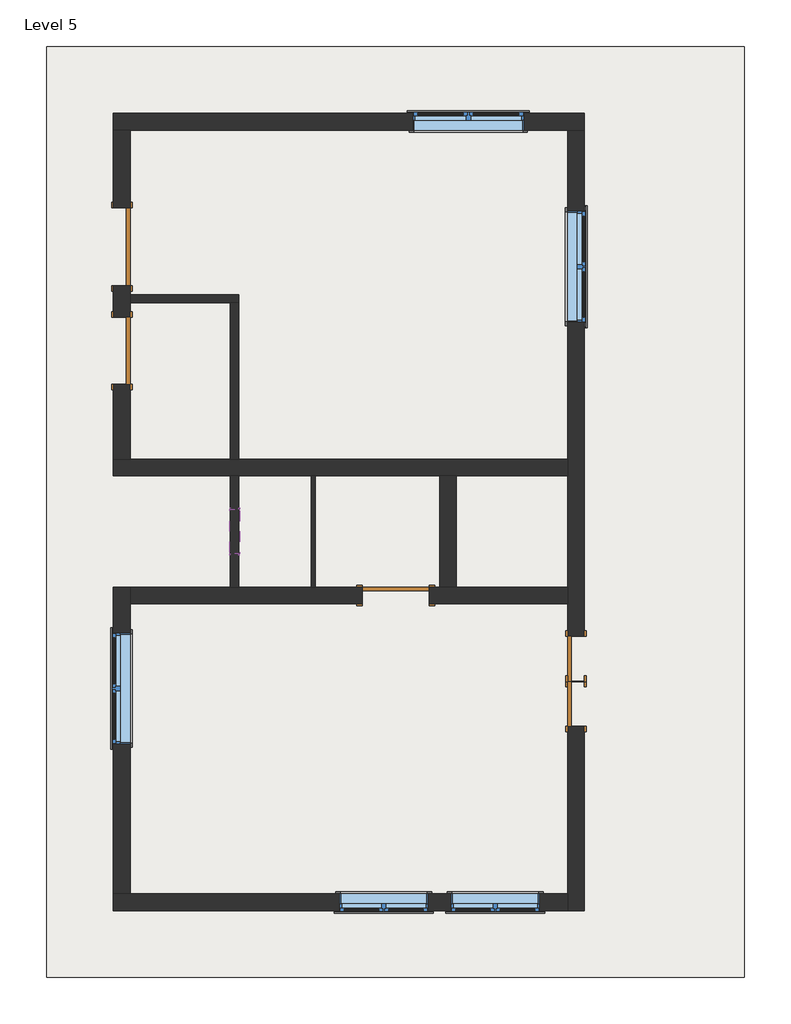
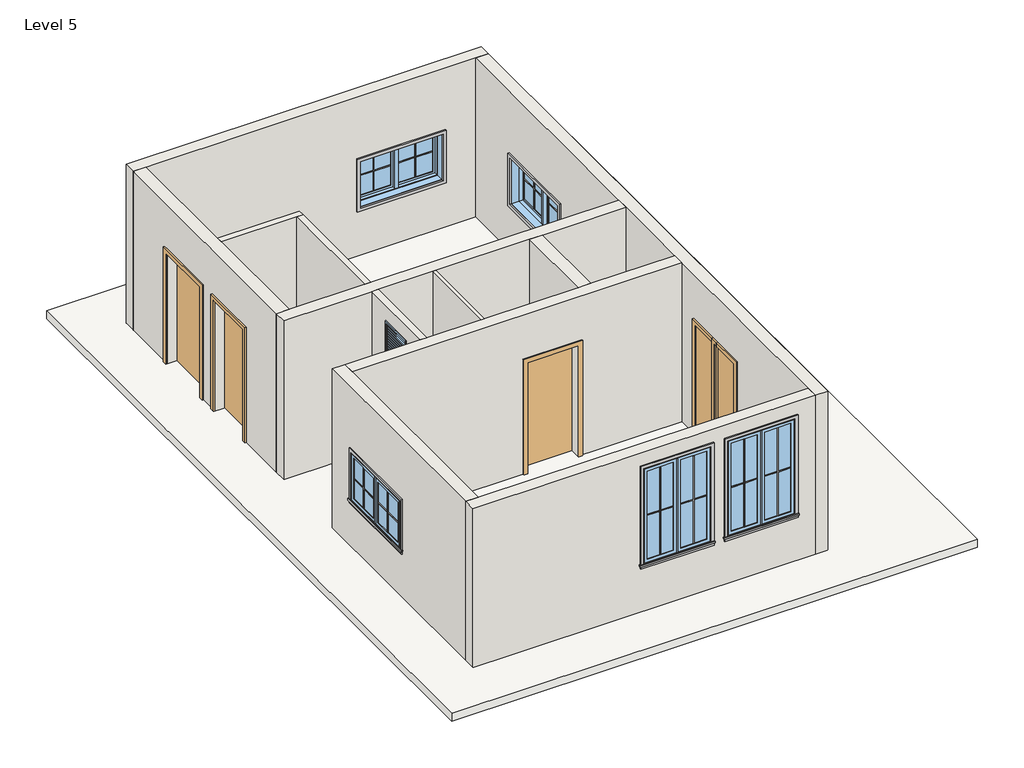
# One storey, incomplete: 20 proxies, 12 walls, 6 windows, 5 doors, 1 roof.
"""IFC4 building model written with IfcOpenShell, lengths in millimetres."""

from ifc_helpers import new_model, si_unit, frame, origin, place, context, project, spatial, polyline, outline, extrude, faceted_brep, transform, mapped, element, save
from components import muntin_pattern_2x2_muntin_pattern_2x2_9352d081, muntin_pattern_2x2_muntin_pattern_2x2_5c2cbe28, muntin_pattern_2x2_muntin_pattern_2x2_2b4d9f72, muntin_pattern_2x2_muntin_pattern_2x2_ef995ed3, trim_window_exterior_flat_with_sill_979bde60, trim_window_exterior_flat_with_sill_b7e4d11c, trim_window_interior_flat_picture_frame_7883d11b, trim_window_interior_flat_picture_frame_936b8d2a, single_flush_door_2_0d3b4037, single_flush_door_2_4a3212df, door_a90ba1ad, door_0ca8825f, door_9d399b00, window_casement_double_c1d95f0f, window_casement_double_wall_4_6ca1769e, window_d39e7ecb

model = new_model("IFC4")

# Units and contexts
model_context = context("Model", 3, world=origin())
ifc_project = project(units=[si_unit("LENGTHUNIT", "METRE", prefix="MILLI")], contexts=[model_context])

# Site, building, storey
site = spatial("IfcSite", under=ifc_project)
building = spatial("IfcBuilding", under=site)
storey = spatial("IfcBuildingStorey", under=building, Name="Level 5", Elevation=9601.2)

# Proxies
placement = place(None, origin())
muntin_pattern_2x2_muntin_pattern_2x2_shape = muntin_pattern_2x2_muntin_pattern_2x2_9352d081(model_context)
element("IfcBuildingElementProxy", 1, Name="Muntin Pattern_2x2 : Muntin Pattern_2x2", ObjectType="Muntin Pattern_2x2 : Muntin Pattern_2x2", at=placement, inside=storey, context=model_context, shape_type="MappedRepresentation", body=[
    mapped(muntin_pattern_2x2_muntin_pattern_2x2_shape, transform((-4785.3510342, -2707.8617544, 10585.45), x_axis=(0.0, 1.0, 0.0), y_axis=(-1.0, 0.0, 0.0), z_axis=(0.0, 0.0, 1.0))),
])
element("IfcBuildingElementProxy", 2, Name="Muntin Pattern_2x2 : Muntin Pattern_2x2", ObjectType="Muntin Pattern_2x2 : Muntin Pattern_2x2", at=placement, inside=storey, context=model_context, shape_type="MappedRepresentation", body=[
    mapped(muntin_pattern_2x2_muntin_pattern_2x2_shape, transform((1634.4989658, 3816.7632456, 10585.45), x_axis=(0.0, -1.0, 0.0), y_axis=(1.0, 0.0, 0.0), z_axis=(0.0, 0.0, 1.0))),
])
element("IfcBuildingElementProxy", 3, Name="Muntin Pattern_2x2 : Muntin Pattern_2x2", ObjectType="Muntin Pattern_2x2 : Muntin Pattern_2x2", at=placement, inside=storey, context=model_context, shape_type="MappedRepresentation", body=[
    mapped(muntin_pattern_2x2_muntin_pattern_2x2_shape, transform((-322.8885342, 5523.3257456, 10585.45), x_axis=(1.0, 0.0, 0.0), y_axis=(0.0, 1.0, 0.0), z_axis=(0.0, 0.0, 1.0))),
])
muntin_pattern_2x2_muntin_pattern_2x2_2_shape = muntin_pattern_2x2_muntin_pattern_2x2_5c2cbe28(model_context)
element("IfcBuildingElementProxy", 4, Name="Muntin Pattern_2x2 : Muntin Pattern_2x2", ObjectType="Muntin Pattern_2x2 : Muntin Pattern_2x2", at=placement, inside=storey, context=model_context, shape_type="MappedRepresentation", body=[
    mapped(muntin_pattern_2x2_muntin_pattern_2x2_2_shape, transform((-4785.3510342, -1949.0367544, 10585.45), x_axis=(0.0, -1.0, 0.0), y_axis=(1.0, 0.0, 0.0), z_axis=(0.0, 0.0, 1.0))),
])
element("IfcBuildingElementProxy", 5, Name="Muntin Pattern_2x2 : Muntin Pattern_2x2", ObjectType="Muntin Pattern_2x2 : Muntin Pattern_2x2", at=placement, inside=storey, context=model_context, shape_type="MappedRepresentation", body=[
    mapped(muntin_pattern_2x2_muntin_pattern_2x2_2_shape, transform((1634.4989658, 3057.9382456, 10585.45), x_axis=(0.0, 1.0, 0.0), y_axis=(-1.0, 0.0, 0.0), z_axis=(0.0, 0.0, 1.0))),
])
element("IfcBuildingElementProxy", 6, Name="Muntin Pattern_2x2 : Muntin Pattern_2x2", ObjectType="Muntin Pattern_2x2 : Muntin Pattern_2x2", at=placement, inside=storey, context=model_context, shape_type="MappedRepresentation", body=[
    mapped(muntin_pattern_2x2_muntin_pattern_2x2_2_shape, transform((435.9364658, 5523.3257456, 10585.45), x_axis=(-1.0, 0.0, 0.0), y_axis=(0.0, -1.0, 0.0), z_axis=(0.0, 0.0, 1.0))),
])
muntin_pattern_2x2_muntin_pattern_2x2_3_shape = muntin_pattern_2x2_muntin_pattern_2x2_2b4d9f72(model_context)
element("IfcBuildingElementProxy", 7, Name="Muntin Pattern_2x2 : Muntin Pattern_2x2", ObjectType="Muntin Pattern_2x2 : Muntin Pattern_2x2", at=placement, inside=storey, context=model_context, shape_type="MappedRepresentation", body=[
    mapped(muntin_pattern_2x2_muntin_pattern_2x2_3_shape, transform((-795.9635342, -5354.2242544, 10585.45), x_axis=(-1.0, 0.0, 0.0), y_axis=(0.0, -1.0, 0.0), z_axis=(0.0, 0.0, 1.0))),
])
element("IfcBuildingElementProxy", 8, Name="Muntin Pattern_2x2 : Muntin Pattern_2x2", ObjectType="Muntin Pattern_2x2 : Muntin Pattern_2x2", at=placement, inside=storey, context=model_context, shape_type="MappedRepresentation", body=[
    mapped(muntin_pattern_2x2_muntin_pattern_2x2_3_shape, transform((728.0364658, -5354.2242544, 10585.45), x_axis=(-1.0, 0.0, 0.0), y_axis=(0.0, -1.0, 0.0), z_axis=(0.0, 0.0, 1.0))),
])
muntin_pattern_2x2_muntin_pattern_2x2_4_shape = muntin_pattern_2x2_muntin_pattern_2x2_ef995ed3(model_context)
element("IfcBuildingElementProxy", 9, Name="Muntin Pattern_2x2 : Muntin Pattern_2x2", ObjectType="Muntin Pattern_2x2 : Muntin Pattern_2x2", at=placement, inside=storey, context=model_context, shape_type="MappedRepresentation", body=[
    mapped(muntin_pattern_2x2_muntin_pattern_2x2_4_shape, transform((-1402.3885342, -5354.2242544, 10585.45), x_axis=(1.0, 0.0, 0.0), y_axis=(0.0, 1.0, 0.0), z_axis=(0.0, 0.0, 1.0))),
])
element("IfcBuildingElementProxy", 10, Name="Muntin Pattern_2x2 : Muntin Pattern_2x2", ObjectType="Muntin Pattern_2x2 : Muntin Pattern_2x2", at=placement, inside=storey, context=model_context, shape_type="MappedRepresentation", body=[
    mapped(muntin_pattern_2x2_muntin_pattern_2x2_4_shape, transform((121.6114658, -5354.2242544, 10585.45), x_axis=(1.0, 0.0, 0.0), y_axis=(0.0, 1.0, 0.0), z_axis=(0.0, 0.0, 1.0))),
])
trim_window_exterior_flat_with_sill_shape = trim_window_exterior_flat_with_sill_979bde60(model_context)
element("IfcBuildingElementProxy", 11, Name="Trim-Window-Exterior-Flat : with Sill", ObjectType="Trim-Window-Exterior-Flat : with Sill", at=placement, inside=storey, context=model_context, shape_type="MappedRepresentation", body=[
    mapped(trim_window_exterior_flat_with_sill_shape, transform((-4794.8760342, -2328.4492544, 11430.0), x_axis=(0.0, -1.0, 0.0), y_axis=(0.0, 0.0, 1.0), z_axis=(-1.0, 0.0, 0.0))),
])
element("IfcBuildingElementProxy", 12, Name="Trim-Window-Exterior-Flat : with Sill", ObjectType="Trim-Window-Exterior-Flat : with Sill", at=placement, inside=storey, context=model_context, shape_type="MappedRepresentation", body=[
    mapped(trim_window_exterior_flat_with_sill_shape, transform((1644.0239658, 3437.3507456, 11430.0), x_axis=(0.0, 1.0, 0.0), y_axis=(0.0, 0.0, 1.0), z_axis=(1.0, 0.0, 0.0))),
])
element("IfcBuildingElementProxy", 13, Name="Trim-Window-Exterior-Flat : with Sill", ObjectType="Trim-Window-Exterior-Flat : with Sill", at=placement, inside=storey, context=model_context, shape_type="MappedRepresentation", body=[
    mapped(trim_window_exterior_flat_with_sill_shape, transform((56.5239658, 5532.8507456, 11430.0), x_axis=(-1.0, 0.0, 0.0), y_axis=(0.0, 0.0, 1.0), z_axis=(0.0, 1.0, 0.0))),
])
trim_window_exterior_flat_with_sill_2_shape = trim_window_exterior_flat_with_sill_b7e4d11c(model_context)
element("IfcBuildingElementProxy", 14, Name="Trim-Window-Exterior-Flat : with Sill", ObjectType="Trim-Window-Exterior-Flat : with Sill", at=placement, inside=storey, context=model_context, shape_type="MappedRepresentation", body=[
    mapped(trim_window_exterior_flat_with_sill_2_shape, transform((-1099.1760342, -5363.7492544, 12344.4), x_axis=(1.0, 0.0, 0.0), y_axis=(0.0, 0.0, 1.0), z_axis=(0.0, -1.0, 0.0))),
])
element("IfcBuildingElementProxy", 15, Name="Trim-Window-Exterior-Flat : with Sill", ObjectType="Trim-Window-Exterior-Flat : with Sill", at=placement, inside=storey, context=model_context, shape_type="MappedRepresentation", body=[
    mapped(trim_window_exterior_flat_with_sill_2_shape, transform((424.8239658, -5363.7492544, 12344.4), x_axis=(1.0, 0.0, 0.0), y_axis=(0.0, 0.0, 1.0), z_axis=(0.0, -1.0, 0.0))),
])
trim_window_interior_flat_picture_frame_shape = trim_window_interior_flat_picture_frame_7883d11b(model_context)
element("IfcBuildingElementProxy", 16, Name="Trim-Window-Interior-Flat : Picture Frame", ObjectType="Trim-Window-Interior-Flat : Picture Frame", at=placement, inside=storey, context=model_context, shape_type="MappedRepresentation", body=[
    mapped(trim_window_interior_flat_picture_frame_shape, transform((-4566.2760342, -2328.4492544, 11430.0), x_axis=(0.0, 1.0, 0.0), y_axis=(0.0, 0.0, 1.0), z_axis=(1.0, 0.0, 0.0))),
])
element("IfcBuildingElementProxy", 17, Name="Trim-Window-Interior-Flat : Picture Frame", ObjectType="Trim-Window-Interior-Flat : Picture Frame", at=placement, inside=storey, context=model_context, shape_type="MappedRepresentation", body=[
    mapped(trim_window_interior_flat_picture_frame_shape, transform((1415.4239658, 3437.3507456, 11430.0), x_axis=(0.0, -1.0, 0.0), y_axis=(0.0, 0.0, 1.0), z_axis=(-1.0, 0.0, 0.0))),
])
element("IfcBuildingElementProxy", 18, Name="Trim-Window-Interior-Flat : Picture Frame", ObjectType="Trim-Window-Interior-Flat : Picture Frame", at=placement, inside=storey, context=model_context, shape_type="MappedRepresentation", body=[
    mapped(trim_window_interior_flat_picture_frame_shape, transform((56.5239658, 5304.2507456, 11430.0), x_axis=(1.0, 0.0, 0.0), y_axis=(0.0, 0.0, 1.0), z_axis=(0.0, -1.0, 0.0))),
])
trim_window_interior_flat_picture_frame_2_shape = trim_window_interior_flat_picture_frame_936b8d2a(model_context)
element("IfcBuildingElementProxy", 19, Name="Trim-Window-Interior-Flat : Picture Frame", ObjectType="Trim-Window-Interior-Flat : Picture Frame", at=placement, inside=storey, context=model_context, shape_type="MappedRepresentation", body=[
    mapped(trim_window_interior_flat_picture_frame_2_shape, transform((-1099.1760342, -5135.1492544, 12344.4), x_axis=(-1.0, 0.0, 0.0), y_axis=(0.0, 0.0, 1.0), z_axis=(0.0, 1.0, 0.0))),
])
element("IfcBuildingElementProxy", 20, Name="Trim-Window-Interior-Flat : Picture Frame", ObjectType="Trim-Window-Interior-Flat : Picture Frame", at=placement, inside=storey, context=model_context, shape_type="MappedRepresentation", body=[
    mapped(trim_window_interior_flat_picture_frame_2_shape, transform((424.8239658, -5135.1492544, 12344.4), x_axis=(-1.0, 0.0, 0.0), y_axis=(0.0, 0.0, 1.0), z_axis=(0.0, 1.0, 0.0))),
])

# Doors
single_flush_door_2_shape = single_flush_door_2_0d3b4037(model_context)
element("IfcDoor", 21, ObjectType="Single-Flush : door 2'", at=placement, inside=storey, context=model_context, shape_type="MappedRepresentation", body=[
    mapped(single_flush_door_2_shape, transform((1529.7239658, -1922.0492544, 9601.2), x_axis=(0.0, 1.0, 0.0), y_axis=(-1.0, 0.0, 0.0), z_axis=(0.0, 0.0, 1.0))),
])
single_flush_door_2_2_shape = single_flush_door_2_4a3212df(model_context)
element("IfcDoor", 22, ObjectType="Single-Flush : door 2'", at=placement, inside=storey, context=model_context, shape_type="MappedRepresentation", body=[
    mapped(single_flush_door_2_2_shape, transform((1529.7239658, -2537.9992544, 9601.2), x_axis=(0.0, -1.0, 0.0), y_axis=(1.0, 0.0, 0.0), z_axis=(0.0, 0.0, 1.0))),
])
door_shape = door_a90ba1ad(model_context)
element("IfcDoor", 23, ObjectType="Single-Flush : door 2'6\"", at=placement, inside=storey, context=model_context, shape_type="MappedRepresentation", body=[
    mapped(door_shape, transform((-4680.5760342, 2288.0007456, 9601.2), x_axis=(0.0, 1.0, 0.0), y_axis=(-1.0, 0.0, 0.0), z_axis=(0.0, 0.0, 1.0))),
])
door_2_shape = door_0ca8825f(model_context)
element("IfcDoor", 24, ObjectType="Single-Flush : door 2'6\"", at=placement, inside=storey, context=model_context, shape_type="MappedRepresentation", body=[
    mapped(door_2_shape, transform((-934.0760342, -1058.4492544, 9601.2), x_axis=(1.0, 0.0, 0.0), y_axis=(0.0, 1.0, 0.0), z_axis=(0.0, 0.0, 1.0))),
])
door_3_shape = door_9d399b00(model_context)
element("IfcDoor", 25, ObjectType="Single-Flush : door 3'6\"", at=placement, inside=storey, context=model_context, shape_type="MappedRepresentation", body=[
    mapped(door_3_shape, transform((-4680.5760342, 3710.4007456, 9601.2), x_axis=(0.0, -1.0, 0.0), y_axis=(1.0, 0.0, 0.0), z_axis=(0.0, 0.0, 1.0))),
])

# Roof
element("IfcRoof", 26, ObjectType="roof 6\"", at=placement, inside=storey, context=model_context, shape_type="SweptSolid", body=[
    extrude(outline(polyline([(-5709.2760342, 6447.2507456), (3828.4239658, 6447.2507456), (3828.4239658, -6278.1492544), (-5709.2760342, -6278.1492544), (-5709.2760342, 6447.2507456)])), frame((0.0, 0.0, 9448.8), z_axis=(0.0, 0.0, 1.0), x_axis=(1.0, 0.0, 0.0)), (0.0, 0.0, 1.0), 152.4),
])

# Walls
element("IfcWall", 27, ObjectType="wall 2\"", at=placement, inside=storey, context=model_context, shape_type="SweptSolid", body=[
    extrude(outline(polyline([(-2089.7760342, -944.1492544), (-2089.7760342, 579.8507456), (-2038.9760342, 579.8507456), (-2038.9760342, -944.1492544), (-2089.7760342, -944.1492544)])), frame((0.0, 0.0, 9601.2), z_axis=(0.0, 0.0, 1.0), x_axis=(1.0, 0.0, 0.0)), (0.0, 0.0, 1.0), 3048.0),
])
element("IfcWall", 28, ObjectType="wall 4.5\"", at=placement, inside=storey, context=model_context, shape_type="Brep", body=[
    faceted_brep([(-4566.2760342, 2942.0507456, 9601.2), (-3194.6760342, 2942.0507456, 9601.2), (-3080.3760342, 2942.0507456, 9601.2), (-3080.3760342, 2942.0507456, 12649.2), (-3194.6760342, 2942.0507456, 12649.2), (-4566.2760342, 2942.0507456, 12649.2), (-4566.2760342, 3056.3507456, 9601.2), (-4566.2760342, 3056.3507456, 12649.2), (-3080.3760342, 3056.3507456, 12649.2), (-3080.3760342, 3056.3507456, 9601.2)], [[[0, 1, 2, 3, 4, 5]], [[6, 7, 8, 9]], [[2, 1, 0, 6, 9]], [[0, 5, 7, 6]], [[3, 2, 9, 8]], [[5, 4, 3, 8, 7]]]),
])
element("IfcWall", 29, ObjectType="wall 4.5\"", at=placement, inside=storey, context=model_context, shape_type="SweptSolid", body=[
    extrude(outline(polyline([(-3194.6760342, 808.4507456), (-3194.6760342, 2942.0507456), (-3080.3760342, 2942.0507456), (-3080.3760342, 808.4507456), (-3194.6760342, 808.4507456)])), frame((0.0, 0.0, 9601.2), z_axis=(0.0, 0.0, 1.0), x_axis=(1.0, 0.0, 0.0)), (0.0, 0.0, 1.0), 3048.0),
])
element("IfcWall", 30, ObjectType="wall 4.5\"", at=placement, inside=storey, context=model_context, shape_type="SweptSolid", body=[
    extrude(outline(polyline([(579.8507456, 9601.2), (-944.1492544, 9601.2), (-944.1492544, 12649.2), (579.8507456, 12649.2), (579.8507456, 9601.2)]), holes=[polyline([(-486.9492544, 12344.4), (-486.9492544, 11734.8), (122.6507456, 11734.8), (122.6507456, 12344.4), (-486.9492544, 12344.4)])]), frame((-3194.6760342, 0.0, 0.0), z_axis=(1.0, 0.0, 0.0), x_axis=(0.0, 1.0, 0.0)), (0.0, 0.0, 1.0), 114.3),
])
element("IfcWall", 31, ObjectType="wall 9\"", at=placement, inside=storey, context=model_context, shape_type="Brep", body=[
    faceted_brep([(-4794.8760342, 5304.2507456, 9601.2), (-4566.2760342, 5304.2507456, 9601.2), (1415.4239658, 5304.2507456, 9601.2), (1644.0239658, 5304.2507456, 9601.2), (1644.0239658, 5304.2507456, 12649.2), (1415.4239658, 5304.2507456, 12649.2), (-4566.2760342, 5304.2507456, 12649.2), (-4794.8760342, 5304.2507456, 12649.2), (818.5239658, 5304.2507456, 11430.0), (818.5239658, 5304.2507456, 10515.6), (-705.4760342, 5304.2507456, 10515.6), (-705.4760342, 5304.2507456, 11430.0), (-4794.8760342, 5532.8507456, 9601.2), (-4794.8760342, 5532.8507456, 12649.2), (1644.0239658, 5532.8507456, 12649.2), (1644.0239658, 5532.8507456, 9601.2), (818.5239658, 5532.8507456, 11430.0), (-705.4760342, 5532.8507456, 11430.0), (-705.4760342, 5532.8507456, 10515.6), (818.5239658, 5532.8507456, 10515.6)], [[[0, 1, 2, 3, 4, 5, 6, 7], [8, 9, 10, 11]], [[12, 13, 14, 15], [16, 17, 18, 19]], [[3, 2, 1, 0, 12, 15]], [[4, 3, 15, 14]], [[0, 7, 13, 12]], [[9, 8, 16, 19]], [[10, 9, 19, 18]], [[11, 10, 18, 17]], [[8, 11, 17, 16]], [[7, 6, 5, 4, 14, 13]]]),
])
element("IfcWall", 32, ObjectType="wall 9\"", at=placement, inside=storey, context=model_context, shape_type="Brep", body=[
    faceted_brep([(1415.4239658, 5304.2507456, 12649.2), (1415.4239658, 5304.2507456, 9601.2), (1415.4239658, 808.4507456, 9601.2), (1415.4239658, 579.8507456, 9601.2), (1415.4239658, -944.1492544, 9601.2), (1415.4239658, -1172.7492544, 9601.2), (1415.4239658, -1617.2492544, 9601.2), (1415.4239658, -1617.2492544, 11734.8), (1415.4239658, -2226.8492544, 11734.8), (1415.4239658, -2226.8492544, 9601.2), (1415.4239658, -2233.1992544, 9601.2), (1415.4239658, -2233.1992544, 11734.8), (1415.4239658, -2842.7992544, 11734.8), (1415.4239658, -2842.7992544, 9601.2), (1415.4239658, -5135.1492544, 9601.2), (1415.4239658, -5363.7492544, 9601.2), (1415.4239658, -5363.7492544, 12649.2), (1415.4239658, -5135.1492544, 12649.2), (1415.4239658, -1172.7492544, 12649.2), (1415.4239658, -944.1492544, 12649.2), (1415.4239658, 579.8507456, 12649.2), (1415.4239658, 808.4507456, 12649.2), (1415.4239658, 2675.3507456, 11430.0), (1415.4239658, 2675.3507456, 10515.6), (1415.4239658, 4199.3507456, 10515.6), (1415.4239658, 4199.3507456, 11430.0), (1644.0239658, 5304.2507456, 9601.2), (1644.0239658, 5304.2507456, 12649.2), (1644.0239658, -5363.7492544, 12649.2), (1644.0239658, -5363.7492544, 9601.2), (1644.0239658, -2842.7992544, 9601.2), (1644.0239658, -2842.7992544, 11734.8), (1644.0239658, -2233.1992544, 11734.8), (1644.0239658, -2233.1992544, 9601.2), (1644.0239658, -2226.8492544, 9601.2), (1644.0239658, -2226.8492544, 11734.8), (1644.0239658, -1617.2492544, 11734.8), (1644.0239658, -1617.2492544, 9601.2), (1644.0239658, 2675.3507456, 11430.0), (1644.0239658, 4199.3507456, 11430.0), (1644.0239658, 4199.3507456, 10515.6), (1644.0239658, 2675.3507456, 10515.6)], [[[0, 1, 2, 3, 4, 5, 6, 7, 8, 9, 10, 11, 12, 13, 14, 15, 16, 17, 18, 19, 20, 21], [22, 23, 24, 25]], [[26, 27, 28, 29, 30, 31, 32, 33, 34, 35, 36, 37], [38, 39, 40, 41]], [[1, 26, 37, 6, 5, 4, 3, 2]], [[29, 15, 14, 13, 30]], [[9, 34, 33, 10]], [[1, 0, 27, 26]], [[16, 15, 29, 28]], [[23, 22, 38, 41]], [[24, 23, 41, 40]], [[25, 24, 40, 39]], [[22, 25, 39, 38]], [[7, 6, 37, 36]], [[8, 7, 36, 35]], [[9, 8, 35, 34]], [[12, 31, 30, 13]], [[31, 12, 11, 32]], [[32, 11, 10, 33]], [[0, 21, 20, 19, 18, 17, 16, 28, 27]]]),
])
element("IfcWall", 33, ObjectType="wall 9\"", at=placement, inside=storey, context=model_context, shape_type="Brep", body=[
    faceted_brep([(1415.4239658, 808.4507456, 9601.2), (-3080.3760342, 808.4507456, 9601.2), (-3194.6760342, 808.4507456, 9601.2), (-4566.2760342, 808.4507456, 9601.2), (-4794.8760342, 808.4507456, 9601.2), (-4794.8760342, 808.4507456, 12649.2), (-4566.2760342, 808.4507456, 12649.2), (-3194.6760342, 808.4507456, 12649.2), (-3080.3760342, 808.4507456, 12649.2), (1415.4239658, 808.4507456, 12649.2), (1415.4239658, 579.8507456, 9601.2), (1415.4239658, 579.8507456, 12649.2), (-108.5760342, 579.8507456, 12649.2), (-337.1760342, 579.8507456, 12649.2), (-2038.9760342, 579.8507456, 12649.2), (-2089.7760342, 579.8507456, 12649.2), (-3080.3760342, 579.8507456, 12649.2), (-3194.6760342, 579.8507456, 12649.2), (-4794.8760342, 579.8507456, 12649.2), (-4794.8760342, 579.8507456, 9601.2), (-3194.6760342, 579.8507456, 9601.2), (-3080.3760342, 579.8507456, 9601.2), (-2089.7760342, 579.8507456, 9601.2), (-2038.9760342, 579.8507456, 9601.2), (-337.1760342, 579.8507456, 9601.2), (-108.5760342, 579.8507456, 9601.2)], [[[0, 1, 2, 3, 4, 5, 6, 7, 8, 9]], [[10, 11, 12, 13, 14, 15, 16, 17, 18, 19, 20, 21, 22, 23, 24, 25]], [[4, 3, 2, 1, 0, 10, 25, 24, 23, 22, 21, 20, 19]], [[0, 9, 11, 10]], [[5, 4, 19, 18]], [[9, 8, 7, 6, 5, 18, 17, 16, 15, 14, 13, 12, 11]]]),
])
element("IfcWall", 34, ObjectType="wall 9\"", at=placement, inside=storey, context=model_context, shape_type="Brep", body=[
    faceted_brep([(-4566.2760342, 2745.2007456, 11734.8), (-4566.2760342, 2745.2007456, 9601.2), (-4566.2760342, 2942.0507456, 9601.2), (-4566.2760342, 3056.3507456, 9601.2), (-4566.2760342, 3177.0007456, 9601.2), (-4566.2760342, 3177.0007456, 11734.8), (-4566.2760342, 4243.8007456, 11734.8), (-4566.2760342, 4243.8007456, 9601.2), (-4566.2760342, 5304.2507456, 9601.2), (-4566.2760342, 5304.2507456, 12649.2), (-4566.2760342, 3056.3507456, 12649.2), (-4566.2760342, 2942.0507456, 12649.2), (-4566.2760342, 808.4507456, 12649.2), (-4566.2760342, 808.4507456, 9601.2), (-4566.2760342, 1830.8007456, 9601.2), (-4566.2760342, 1830.8007456, 11734.8), (-4794.8760342, 3177.0007456, 9601.2), (-4794.8760342, 2745.2007456, 9601.2), (-4794.8760342, 2745.2007456, 11734.8), (-4794.8760342, 1830.8007456, 11734.8), (-4794.8760342, 1830.8007456, 9601.2), (-4794.8760342, 808.4507456, 9601.2), (-4794.8760342, 808.4507456, 12649.2), (-4794.8760342, 5304.2507456, 12649.2), (-4794.8760342, 5304.2507456, 9601.2), (-4794.8760342, 4243.8007456, 9601.2), (-4794.8760342, 4243.8007456, 11734.8), (-4794.8760342, 3177.0007456, 11734.8)], [[[0, 1, 2, 3, 4, 5, 6, 7, 8, 9, 10, 11, 12, 13, 14, 15]], [[16, 17, 18, 19, 20, 21, 22, 23, 24, 25, 26, 27]], [[25, 24, 8, 7]], [[14, 13, 21, 20]], [[4, 3, 2, 1, 17, 16]], [[9, 8, 24, 23]], [[13, 12, 22, 21]], [[5, 4, 16, 27]], [[6, 5, 27, 26]], [[7, 6, 26, 25]], [[18, 17, 1, 0]], [[19, 18, 0, 15]], [[20, 19, 15, 14]], [[12, 11, 10, 9, 23, 22]]]),
])
element("IfcWall", 35, ObjectType="wall 9\"", at=placement, inside=storey, context=model_context, shape_type="Brep", body=[
    faceted_brep([(1415.4239658, -5135.1492544, 9601.2), (-4566.2760342, -5135.1492544, 9601.2), (-4794.8760342, -5135.1492544, 9601.2), (-4794.8760342, -5135.1492544, 12649.2), (-4566.2760342, -5135.1492544, 12649.2), (1415.4239658, -5135.1492544, 12649.2), (-1708.7760342, -5135.1492544, 12344.4), (-1708.7760342, -5135.1492544, 10515.6), (-489.5760342, -5135.1492544, 10515.6), (-489.5760342, -5135.1492544, 12344.4), (-184.7760342, -5135.1492544, 12344.4), (-184.7760342, -5135.1492544, 10515.6), (1034.4239658, -5135.1492544, 10515.6), (1034.4239658, -5135.1492544, 12344.4), (1415.4239658, -5363.7492544, 9601.2), (1415.4239658, -5363.7492544, 12649.2), (-4794.8760342, -5363.7492544, 12649.2), (-4794.8760342, -5363.7492544, 9601.2), (-1708.7760342, -5363.7492544, 12344.4), (-489.5760342, -5363.7492544, 12344.4), (-489.5760342, -5363.7492544, 10515.6), (-1708.7760342, -5363.7492544, 10515.6), (-184.7760342, -5363.7492544, 12344.4), (1034.4239658, -5363.7492544, 12344.4), (1034.4239658, -5363.7492544, 10515.6), (-184.7760342, -5363.7492544, 10515.6)], [[[0, 1, 2, 3, 4, 5], [6, 7, 8, 9], [10, 11, 12, 13]], [[14, 15, 16, 17], [18, 19, 20, 21], [22, 23, 24, 25]], [[2, 1, 0, 14, 17]], [[0, 5, 15, 14]], [[3, 2, 17, 16]], [[7, 6, 18, 21]], [[8, 7, 21, 20]], [[9, 8, 20, 19]], [[6, 9, 19, 18]], [[11, 10, 22, 25]], [[12, 11, 25, 24]], [[13, 12, 24, 23]], [[10, 13, 23, 22]], [[5, 4, 3, 16, 15]]]),
])
element("IfcWall", 36, ObjectType="wall 9\"", at=placement, inside=storey, context=model_context, shape_type="Brep", body=[
    faceted_brep([(-4566.2760342, -5135.1492544, 9601.2), (-4566.2760342, -1172.7492544, 9601.2), (-4566.2760342, -944.1492544, 9601.2), (-4566.2760342, -944.1492544, 12649.2), (-4566.2760342, -1172.7492544, 12649.2), (-4566.2760342, -5135.1492544, 12649.2), (-4566.2760342, -1566.4492544, 11430.0), (-4566.2760342, -1566.4492544, 10515.6), (-4566.2760342, -3090.4492544, 10515.6), (-4566.2760342, -3090.4492544, 11430.0), (-4794.8760342, -5135.1492544, 9601.2), (-4794.8760342, -5135.1492544, 12649.2), (-4794.8760342, -944.1492544, 12649.2), (-4794.8760342, -944.1492544, 9601.2), (-4794.8760342, -1566.4492544, 11430.0), (-4794.8760342, -3090.4492544, 11430.0), (-4794.8760342, -3090.4492544, 10515.6), (-4794.8760342, -1566.4492544, 10515.6)], [[[0, 1, 2, 3, 4, 5], [6, 7, 8, 9]], [[10, 11, 12, 13], [14, 15, 16, 17]], [[2, 1, 0, 10, 13]], [[0, 5, 11, 10]], [[3, 2, 13, 12]], [[7, 6, 14, 17]], [[8, 7, 17, 16]], [[9, 8, 16, 15]], [[6, 9, 15, 14]], [[5, 4, 3, 12, 11]]]),
])
element("IfcWall", 37, ObjectType="wall 9\"", at=placement, inside=storey, context=model_context, shape_type="Brep", body=[
    faceted_brep([(-476.8760342, -1172.7492544, 11734.8), (-476.8760342, -1172.7492544, 9601.2), (1415.4239658, -1172.7492544, 9601.2), (1415.4239658, -1172.7492544, 12649.2), (-4566.2760342, -1172.7492544, 12649.2), (-4566.2760342, -1172.7492544, 9601.2), (-1391.2760342, -1172.7492544, 9601.2), (-1391.2760342, -1172.7492544, 11734.8), (1415.4239658, -944.1492544, 9601.2), (-108.5760342, -944.1492544, 9601.2), (-337.1760342, -944.1492544, 9601.2), (-476.8760342, -944.1492544, 9601.2), (-476.8760342, -944.1492544, 11734.8), (-1391.2760342, -944.1492544, 11734.8), (-1391.2760342, -944.1492544, 9601.2), (-2038.9760342, -944.1492544, 9601.2), (-2089.7760342, -944.1492544, 9601.2), (-3080.3760342, -944.1492544, 9601.2), (-3194.6760342, -944.1492544, 9601.2), (-4566.2760342, -944.1492544, 9601.2), (-4566.2760342, -944.1492544, 12649.2), (-3194.6760342, -944.1492544, 12649.2), (-3080.3760342, -944.1492544, 12649.2), (-2089.7760342, -944.1492544, 12649.2), (-2038.9760342, -944.1492544, 12649.2), (-337.1760342, -944.1492544, 12649.2), (-108.5760342, -944.1492544, 12649.2), (1415.4239658, -944.1492544, 12649.2)], [[[0, 1, 2, 3, 4, 5, 6, 7]], [[8, 9, 10, 11, 12, 13, 14, 15, 16, 17, 18, 19, 20, 21, 22, 23, 24, 25, 26, 27]], [[6, 5, 19, 18, 17, 16, 15, 14]], [[2, 1, 11, 10, 9, 8]], [[5, 4, 20, 19]], [[3, 2, 8, 27]], [[12, 11, 1, 0]], [[13, 12, 0, 7]], [[14, 13, 7, 6]], [[4, 3, 27, 26, 25, 24, 23, 22, 21, 20]]]),
])
element("IfcWall", 38, ObjectType="wall 9\"", at=placement, inside=storey, context=model_context, shape_type="SweptSolid", body=[
    extrude(outline(polyline([(-108.5760342, 579.8507456), (-108.5760342, -944.1492544), (-337.1760342, -944.1492544), (-337.1760342, 579.8507456), (-108.5760342, 579.8507456)])), frame((0.0, 0.0, 9601.2), z_axis=(0.0, 0.0, 1.0), x_axis=(1.0, 0.0, 0.0)), (0.0, 0.0, 1.0), 3048.0),
])

# Windows
window_casement_double_shape = window_casement_double_c1d95f0f(model_context)
element("IfcWindow", 39, ObjectType="Window-Casement-Double", at=placement, inside=storey, context=model_context, shape_type="MappedRepresentation", body=[
    mapped(window_casement_double_shape, transform((-4680.5760342, -2328.4492544, 9601.2), x_axis=(0.0, 1.0, 0.0), y_axis=(-1.0, 0.0, 0.0), z_axis=(0.0, 0.0, 1.0))),
])
element("IfcWindow", 40, ObjectType="Window-Casement-Double", at=placement, inside=storey, context=model_context, shape_type="MappedRepresentation", body=[
    mapped(window_casement_double_shape, transform((1529.7239658, 3437.3507456, 9601.2), x_axis=(0.0, -1.0, 0.0), y_axis=(1.0, 0.0, 0.0), z_axis=(0.0, 0.0, 1.0))),
])
element("IfcWindow", 41, ObjectType="Window-Casement-Double", at=placement, inside=storey, context=model_context, shape_type="MappedRepresentation", body=[
    mapped(window_casement_double_shape, transform((56.5239658, 5418.5507456, 9601.2), x_axis=(1.0, 0.0, 0.0), y_axis=(0.0, 1.0, 0.0), z_axis=(0.0, 0.0, 1.0))),
])
window_casement_double_wall_4_shape = window_casement_double_wall_4_6ca1769e(model_context)
element("IfcWindow", 42, ObjectType="Window-Casement-Double : wall 4'", at=placement, inside=storey, context=model_context, shape_type="MappedRepresentation", body=[
    mapped(window_casement_double_wall_4_shape, transform((-1099.1760342, -5249.4492544, 9601.2), x_axis=(-1.0, 0.0, 0.0), y_axis=(0.0, -1.0, 0.0), z_axis=(0.0, 0.0, 1.0))),
])
element("IfcWindow", 43, ObjectType="Window-Casement-Double : wall 4'", at=placement, inside=storey, context=model_context, shape_type="MappedRepresentation", body=[
    mapped(window_casement_double_wall_4_shape, transform((424.8239658, -5249.4492544, 9601.2), x_axis=(-1.0, 0.0, 0.0), y_axis=(0.0, -1.0, 0.0), z_axis=(0.0, 0.0, 1.0))),
])
window_shape = window_d39e7ecb(model_context)
element("IfcWindow", 44, ObjectType="Window-Louvers : 24\" x 24\"", at=placement, inside=storey, context=model_context, shape_type="MappedRepresentation", body=[
    mapped(window_shape, transform((-3143.8760342, -182.1492544, 10820.4), x_axis=(0.0, 1.0, 0.0), y_axis=(-1.0, 0.0, 0.0), z_axis=(0.0, 0.0, 1.0))),
])

save(model, "model.ifc")

# Revit data of these elements
# Type "Muntin Pattern_2x2 : Muntin Pattern_2x2"
#   Width [instance default] = 4' - 0"
#   Thickness = 0' - 0 1/2"
#   Height [instance default] = 4' - 0"
#   Distance = 0' - 0 3/4"
#   Interior Material [instance default] = none
#   Exterior Material [instance default] = none
#   Default Elevation = 0
# Type "Trim-Window-Exterior-Flat : with Sill"
#   Trim Width = 0' - 2 1/4"
#   Trim Thickness_Picture Frame = 0' - 1 1/4"
#   Trim Thickness_with Sill = 0' - 0 3/4"
#   Sill Thickness = 0' - 1 1/4"
#   Opening Width [instance default] = 2' - 0"
#   Opening Height [instance default] = 3' - 0"
#   Default Elevation = 4' - 0"
#   Sill = yes
#   Picture Frame = no
#   Trim Material [instance default] = none
# Type "Trim-Window-Interior-Flat : Picture Frame"
#   Trim Thickness_Picture Frame = 0' - 1 1/4"
#   Trim Width = 0' - 2 1/4"
#   Trim Thickness_with Sill = 0' - 0 3/4"
#   Sill Thickness = 0' - 1 1/4"
#   Opening Width [instance default] = 2' - 0"
#   Opening Height [instance default] = 3' - 0"
#   Default Elevation = 4' - 0"
#   Sill = no
#   Picture Frame = yes
#   Trim Material [instance default] = none
# Type "Single-Flush : door 2'"
#   Type Mark = "11"
#   Construction Type Id = "MDOOR"
#   Assembly Code = "C1020"
#   Analytic Construction = "Metal"
#   Thickness = 0' - 2"
#   Heat Transfer Coefficient (U) = 0.651978 BTU/(h·ft²·°F)
#   Height = 7' - 0"
#   Trim Projection Ext = 0' - 1"
#   Trim Projection Int = 0' - 1"
#   Trim Width = 0' - 3"
#   Width = 2' - 0"
#   Define Thermal Properties by = 1
#   Door Material = Door - Panel
#   Frame Material = Door - Frame
#   Visual Light Transmittance = 0
#   Solar Heat Gain Coefficient = 0
#   Function = (empty or 0)
#   Wall Closure = (empty or 0)
# Type "Single-Flush : door 2'6\""
#   Type Mark = "8"
#   Construction Type Id = "MDOOR"
#   Assembly Code = "C1020"
#   Analytic Construction = "Metal"
#   Thickness = 0' - 2"
#   Heat Transfer Coefficient (U) = 0.651978 BTU/(h·ft²·°F)
#   Height = 7' - 0"
#   Trim Projection Ext = 0' - 1"
#   Trim Projection Int = 0' - 1"
#   Trim Width = 0' - 3"
#   Width = 3' - 0"
#   Define Thermal Properties by = 1
#   Door Material = Door - Panel
#   Frame Material = Door - Frame
#   Visual Light Transmittance = 0
#   Solar Heat Gain Coefficient = 0
#   Function = (empty or 0)
#   Wall Closure = (empty or 0)
# Type "Single-Flush : door 3'6\""
#   Type Mark = "10"
#   Construction Type Id = "MDOOR"
#   Assembly Code = "C1020"
#   Analytic Construction = "Metal"
#   Thickness = 0' - 2"
#   Heat Transfer Coefficient (U) = 0.651978 BTU/(h·ft²·°F)
#   Height = 7' - 0"
#   Trim Projection Ext = 0' - 1"
#   Trim Projection Int = 0' - 1"
#   Trim Width = 0' - 3"
#   Width = 3' - 6"
#   Define Thermal Properties by = 1
#   Door Material = Door - Panel
#   Frame Material = Door - Frame
#   Visual Light Transmittance = 0
#   Solar Heat Gain Coefficient = 0
#   Function = (empty or 0)
#   Wall Closure = (empty or 0)
# Type "roof 6\""
#   Assembly Code = "B1020"
#   Layers, outside or top first: 0' - 6" no material (function 1)
# Type "wall 2\""
#   Assembly Code = "B2010"
#   Layers, outside or top first: 0' - 2" no material (function 1)
# Type "wall 4.5\""
#   Assembly Code = "B2010"
#   Layers, outside or top first: 0' - 4 1/2" no material (function 1)
# Type "wall 9\""
#   Assembly Code = "B2010"
#   Layers, outside or top first: 0' - 9" no material (function 1)
# Type "Window-Casement-Double"
#   Type Mark = "18"
#   Fire Rating = "0.5h"
#   Assembly Code = "B2020100"
#   Analytic Construction = "Double glazing - domestic"
#   Frame Extension [instance default] = 0' - 0 1/4"
#   Window Inset [instance default] = 0' - 0"
#   Wall Thickness [instance default] = 0' - 6"
#   Interior Wall Closure [instance default] = 0' - 2 1/4"
#   Half Width = 2' - 6"
#   Visual Light Transmittance = 0.81
#   Thermal Resistance (R) = 1.8146 (h·ft²·°F)/BTU
#   Solar Heat Gain Coefficient = 0.76
#   Rough Width = 5' - 0 1/2"
#   Rough Height = 3' - 0 1/2"
#   Height = 3' - 0"
#   Heat Transfer Coefficient (U) = 0.5511 BTU/(h·ft²·°F)
#   Exterior Wall Closure [instance default] = 0' - 1 1/4"
#   Extension Jamb [instance default] = 0' - 2 1/4"
#   Default Sill Height = 3' - 0"
#   Width = 5' - 0"
#   Muntin Visibility = yes
#   Interior Trim Visibility [instance default] = yes
#   Exterior Trim Visibility [instance default] = yes
#   Extension Jamb Visibility [instance default] = yes
#   Interior Trim Material = Wood - Stained
#   Muntin Pattern = Muntin Pattern_2x2 : Muntin Pattern_2x2
#   Interior Trim = Trim-Window-Interior-Flat : Picture Frame
#   Interior Frame Material = Wood - Stained
#   Glass Panel Material = Glass
#   Exterior Trim Material = Clad - White
#   Exterior Trim = Trim-Window-Exterior-Flat : with Sill
#   Exterior Frame Material = Clad - White
#   Wall Closure = (empty or 0)
# Type "Window-Casement-Double : wall 4'"
#   Type Mark = "19"
#   Fire Rating = "0.5h"
#   Assembly Code = "B2020100"
#   Analytic Construction = "Double glazing - domestic"
#   Frame Extension [instance default] = 0' - 0 1/4"
#   Window Inset [instance default] = 0' - 0"
#   Wall Thickness [instance default] = 0' - 6"
#   Interior Wall Closure [instance default] = 0' - 2 1/4"
#   Half Width = 2' - 0"
#   Visual Light Transmittance = 0.81
#   Thermal Resistance (R) = 1.8146 (h·ft²·°F)/BTU
#   Solar Heat Gain Coefficient = 0.76
#   Rough Width = 4' - 0 1/2"
#   Rough Height = 6' - 0 1/2"
#   Height = 6' - 0"
#   Heat Transfer Coefficient (U) = 0.5511 BTU/(h·ft²·°F)
#   Exterior Wall Closure [instance default] = 0' - 1 1/4"
#   Extension Jamb [instance default] = 0' - 2 1/4"
#   Default Sill Height = 3' - 0"
#   Width = 4' - 0"
#   Muntin Visibility = yes
#   Interior Trim Visibility [instance default] = yes
#   Exterior Trim Visibility [instance default] = yes
#   Extension Jamb Visibility [instance default] = yes
#   Interior Trim Material = Wood - Stained
#   Muntin Pattern = Muntin Pattern_2x2 : Muntin Pattern_2x2
#   Interior Trim = Trim-Window-Interior-Flat : Picture Frame
#   Interior Frame Material = Wood - Stained
#   Glass Panel Material = Glass
#   Exterior Trim Material = Clad - White
#   Exterior Trim = Trim-Window-Exterior-Flat : with Sill
#   Exterior Frame Material = Clad - White
#   Wall Closure = (empty or 0)
# Type "Window-Louvers : 24\" x 24\""
#   Type Mark = "20"
#   Construction Type Id = "GSP4R"
#   Assembly Code = "B20"
#   Analytic Construction = "1/8 in Pilkington single glazing"
#   Visual Light Transmittance = 0.9
#   Thermal Resistance (R) = 1.53941 (h·ft²·°F)/BTU
#   Solar Heat Gain Coefficient = 0.78
#   Max Height = 1' - 11.74264"
#   Height = 2' - 0"
#   Heat Transfer Coefficient (U) = 0.6496 BTU/(h·ft²·°F)
#   Blade Width [instance default] = 1' - 10 1/2"
#   Blade Vertical Thickness = 0' - 0.35355"
#   Blade Thickness = 0' - 0 1/4"
#   Blade Spacing = 0' - 1 1/2"
#   Blade Height = 0' - 1.85355"
#   Blade Depth = 0' - 3"
#   Blade Angle = 45.00°
#   Default Sill Height = 3' - 0"
#   Trim Projection_Exterior = 0' - 0 1/2"
#   Trim Projection_Interior = 0' - 0 1/2"
#   Trim Width_Exterior = 0' - 1 1/2"
#   Trim Width_Interior = 0' - 1 1/2"
#   Width = 2' - 0"
#   Max Blade Count = 12
#   Define Thermal Properties by = 1
#   Blade Count = 12
#   Frame Material = Birch
#   Louver Material = Birch
#   Trim Exterior Material = Birch
#   Trim Interior Material = Birch
#   Wall Closure = (empty or 0)
# Elements 1, 2, 3, 4, 5, 6 (IfcBuildingElementProxy, "Muntin Pattern_2x2 : Muntin Pattern_2x2")
#   Width = 2' - 0 5/8"
#   Height = 2' - 6 1/2"
#   Interior Material = Wood - Stained
#   Exterior Material = Clad - White
#   Phase Created = New Construction
#   Materials on its faces: "Clad - White", "Wood - Stained"
# Elements 7, 8, 9, 10 (IfcBuildingElementProxy, "Muntin Pattern_2x2 : Muntin Pattern_2x2")
#   Width = 1' - 6 5/8"
#   Height = 5' - 6 1/2"
#   Interior Material = Wood - Stained
#   Exterior Material = Clad - White
#   Phase Created = New Construction
#   Materials on its faces: "Clad - White", "Wood - Stained"
# Elements 11, 12, 13 (IfcBuildingElementProxy, "Trim-Window-Exterior-Flat : with Sill")
#   Opening Width = 5' - 0"
#   Opening Height = 3' - 0"
#   Trim Material = Clad - White
#   Phase Created = New Construction
#   Materials on its faces: "Clad - White"
# Elements 14, 15 (IfcBuildingElementProxy, "Trim-Window-Exterior-Flat : with Sill")
#   Opening Width = 4' - 0"
#   Opening Height = 6' - 0"
#   Trim Material = Clad - White
#   Phase Created = New Construction
#   Materials on its faces: "Clad - White"
# Elements 16, 17, 18 (IfcBuildingElementProxy, "Trim-Window-Interior-Flat : Picture Frame")
#   Opening Width = 5' - 0"
#   Opening Height = 3' - 0"
#   Trim Material = Wood - Stained
#   Phase Created = New Construction
#   Materials on its faces: "Wood - Stained"
# Elements 19, 20 (IfcBuildingElementProxy, "Trim-Window-Interior-Flat : Picture Frame")
#   Opening Width = 4' - 0"
#   Opening Height = 6' - 0"
#   Trim Material = Wood - Stained
#   Phase Created = New Construction
#   Materials on its faces: "Wood - Stained"
# Elements 21, 22 (IfcDoor, "Single-Flush : door 2'")
#   Phase Created = New Construction
#   Materials on its faces: "Door - Frame", "Door - Panel"
# Elements 23, 24 (IfcDoor, "Single-Flush : door 2'6\"")
#   Phase Created = New Construction
#   Materials on its faces: "Door - Frame", "Door - Panel"
# Element 25 (IfcDoor, "Single-Flush : door 3'6\"")
#   Phase Created = New Construction
#   Materials on its faces: "Door - Frame", "Door - Panel"
# Element 26 (IfcRoof, "roof 6\"")
#   built-in parameter 1001705 = 31.5 (stored number, unit not read)
#   built-in parameter 1001701 = -0.5 (stored number, unit not read)
#   built-in parameter 1001710 = 33615
#   Phase Created = New Construction
#   Materials on its faces: "Copper", "Default Roof", "Wood - Stained"
# Element 27 (IfcWall, "wall 2\"")
#   Top Offset = 0' - 0"
#   Base Offset = 0' - 0"
#   Unconnected Height = 10' - 0"
#   wall height = 10' - 0"
#   Phase Created = New Construction
#   Base Constraint = Level 5
#   Materials on its faces: "Default Wall"
# Elements 28, 29 (IfcWall, "wall 4.5\"")
#   Top Offset = 0' - 0"
#   Base Offset = 0' - 0"
#   Unconnected Height = 10' - 0"
#   wall height = 10' - 0"
#   Phase Created = New Construction
#   Base Constraint = Level 5
#   Materials on its faces: "Default Wall"
# Element 30 (IfcWall, "wall 4.5\"")
#   Top Offset = 0' - 0"
#   Base Offset = 0' - 0"
#   Unconnected Height = 10' - 0"
#   wall height = 10' - 0"
#   Phase Created = New Construction
#   Base Constraint = Level 5
#   Materials on its faces: "Default Wall", "Wood Planks"
# Elements 31, 32, 33, 35, 36, 37 (IfcWall, "wall 9\"")
#   Top Offset = 0' - 0"
#   Base Offset = 0' - 0"
#   Unconnected Height = 10' - 0"
#   wall height = 10' - 0"
#   Phase Created = New Construction
#   Base Constraint = Level 5
#   Materials on its faces: "Default Wall", "Wood Planks"
# Element 34 (IfcWall, "wall 9\"")
#   Top Offset = 0' - 0"
#   Base Offset = 0' - 0"
#   Unconnected Height = 10' - 0"
#   wall height = 10' - 0"
#   Phase Created = New Construction
#   Base Constraint = Level 5
#   Materials on its faces: "Default Wall", "Copper", "Wood Planks"
# Element 38 (IfcWall, "wall 9\"")
#   Top Offset = 0' - 0"
#   Base Offset = 0' - 0"
#   Unconnected Height = 10' - 0"
#   wall height = 10' - 0"
#   Phase Created = New Construction
#   Base Constraint = Level 5
#   Materials on its faces: "Default Wall"
# Element 39 (IfcWindow, "Window-Casement-Double")
#   Mark = "19"
#   Window Inset = 0' - 0"
#   Interior Wall Closure = 0' - 2 1/4"
#   Frame Extension = 0' - 0 1/4"
#   Exterior Wall Closure = 0' - 1 1/4"
#   Interior Trim Visibility = yes
#   Exterior Trim Visibility = yes
#   Phase Created = New Construction
#   Materials on its faces: "Wood - Stained", "Glass", "Clad - White"
# Element 40 (IfcWindow, "Window-Casement-Double")
#   Mark = "20"
#   Window Inset = 0' - 0"
#   Interior Wall Closure = 0' - 2 1/4"
#   Frame Extension = 0' - 0 1/4"
#   Exterior Wall Closure = 0' - 1 1/4"
#   Interior Trim Visibility = yes
#   Exterior Trim Visibility = yes
#   Phase Created = New Construction
#   Materials on its faces: "Wood - Stained", "Glass", "Clad - White"
# Element 41 (IfcWindow, "Window-Casement-Double")
#   Mark = "21"
#   Window Inset = 0' - 0"
#   Interior Wall Closure = 0' - 2 1/4"
#   Frame Extension = 0' - 0 1/4"
#   Exterior Wall Closure = 0' - 1 1/4"
#   Interior Trim Visibility = yes
#   Exterior Trim Visibility = yes
#   Phase Created = New Construction
#   Materials on its faces: "Wood - Stained", "Glass", "Clad - White"
# Element 42 (IfcWindow, "Window-Casement-Double : wall 4'")
#   Mark = "22"
#   Window Inset = 0' - 0"
#   Interior Wall Closure = 0' - 2 1/4"
#   Frame Extension = 0' - 0 1/4"
#   Exterior Wall Closure = 0' - 1 1/4"
#   Interior Trim Visibility = yes
#   Exterior Trim Visibility = yes
#   Phase Created = New Construction
#   Materials on its faces: "Wood - Stained", "Glass", "Clad - White"
# Element 43 (IfcWindow, "Window-Casement-Double : wall 4'")
#   Mark = "23"
#   Window Inset = 0' - 0"
#   Interior Wall Closure = 0' - 2 1/4"
#   Frame Extension = 0' - 0 1/4"
#   Exterior Wall Closure = 0' - 1 1/4"
#   Interior Trim Visibility = yes
#   Exterior Trim Visibility = yes
#   Phase Created = New Construction
#   Materials on its faces: "Wood - Stained", "Glass", "Clad - White"
# Element 44 (IfcWindow, "Window-Louvers : 24\" x 24\"")
#   Mark = "24"
#   Blade Width = 1' - 10 1/2"
#   Phase Created = New Construction
#   Materials on its faces: "Birch"
# Materials
#   "Door - Panel": class "Wood", colour RGB 210 159 95, transparency 0, Cost = 0
#   "Door - Frame": colour RGB 118 70 51, transparency 0, Cost = 0
#   "Wood - Stained": class "Wood", colour RGB 224 178 126, transparency 0, Cost = 0
#   "Glass": class "Glass", colour RGB 0 128 192, transparency 0.75, Description = "Soda Lime Glass", Cost = 0
#   "Clad - White": class "Wood", colour RGB 242 242 238, transparency 0, Cost = 0
#   "Birch": class "Wood", colour RGB 224 178 126, transparency 0, Description = "Betula Alleghaniensis", Cost = 0
#   "Copper": class "Metal", colour RGB 0 0 0, transparency 0, Description = "Copper, matte finish", Cost = 0
#   "Default Roof": colour RGB 88 101 114, transparency 0, Cost = 0
#   "Default Wall": colour RGB 128 128 128, transparency 0, Cost = 0
#   "Wood Planks": class "Wood", colour RGB 193 160 115, transparency 0, Description = "Physical material.", Cost = 0
